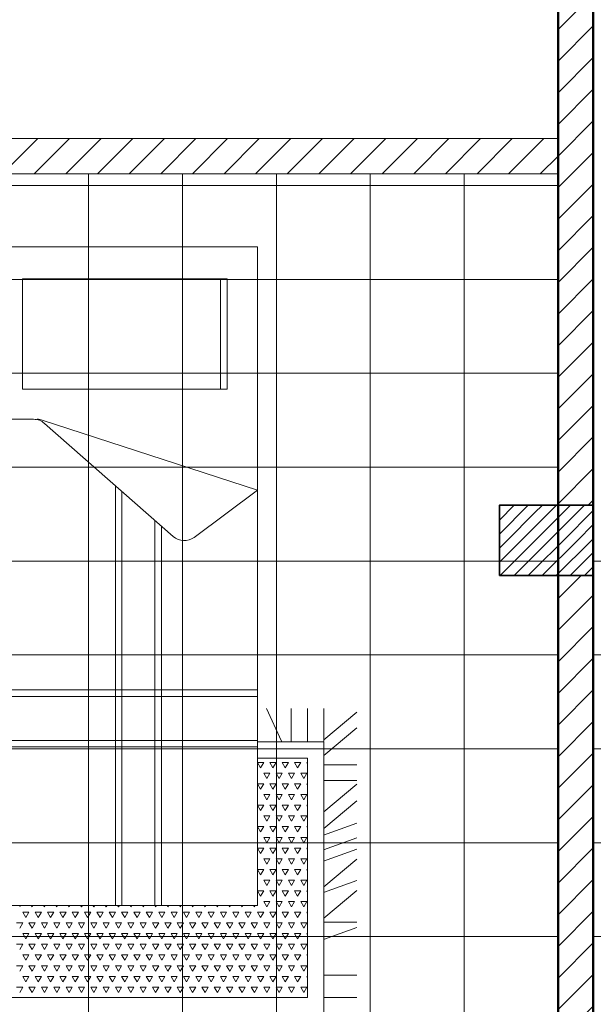
# Model space of a CAD drawing. Units: millimetres. Extents: x 225995 to 227247, y 225507 to 226008.
# Tile 15 of 23: x 226821 to 226894, y 225755 to 225881. Entities that reach past the tile are written whole.
import ezdxf

# ---------------------------------------------------------------- set-up
doc = ezdxf.new("R2010")
doc.units = ezdxf.units.MM
for name, color, linetype, lineweight in [('A-COLS', 40, 'Continuous', 35), ('A-FLOR-PATT', 8, 'Continuous', 13), ('A-FURN', 9, 'Continuous', 18), ('A-WALL', 7, 'Continuous', 50), ('A-WALL-PATT', 8, 'Continuous', 13)]:
    doc.layers.add(name, color=color, linetype=linetype, lineweight=lineweight)
pattern_1 = [(45, (502.0463, 119.0671), (-0.898025612, 0.898025612), [])]

# ---------------------------------------------------------------- blocks, each defined once
blk = doc.blocks.new('A$C6D2A2628')
for p, q in [((0.291, 2.4297), (1.791, 2.4297)), ((1.791, 2.4297), (1.791, 0.4297)), ((1.0779, 2.3321), (1.6991, 2.3321)), ((1.0779, 1.9967), (1.0779, 2.3321)), ((1.6791, 2.3321), (1.6791, 1.9967)), ((1.6991, 2.3321), (1.6991, 1.9967)), ((1.6991, 1.9967), (1.0779, 1.9967)), ((0.9515, 1.9058), (1.1116, 1.9058)), ((1.791, 1.6908), (1.138, 1.9034)), ((1.1446, 1.8934), (1.5358, 1.5497)), ((1.3599, 1.7043), (1.3599, 0.4297)), ((1.3799, 1.6867), (1.3799, 0.4297)), ((1.5987, 1.5472), (1.791, 1.6908)), ((1.4799, 1.5988), (1.4799, 0.4297)), ((1.4999, 1.5812), (1.4999, 0.4297)), ((0.291, 1.0837), (1.791, 1.0837)), ((0.291, 1.0637), (1.791, 1.0637)), ((1.8187, 1.0278), (1.8641, 0.9278)), ((1.8932, 1.0278), (1.8932, 0.9278)), ((1.9432, 1.0278), (1.9432, 0.9278)), ((1.9932, 1.0278), (1.9932, 0.9278)), ((1.9932, 0.9324), (2.0932, 1.016)), ((1.9932, 0.8849), (2.0932, 0.9685)), ((0.291, 0.9307), (1.791, 0.9307)), ((0.291, 0.9107), (1.791, 0.9107)), ((1.9932, 0.9267), (1.791, 0.9267)), ((1.9932, 0.1), (1.9932, 0.9267)), ((1.9432, 0.8767), (1.791, 0.8767)), ((1.9432, 0.15), (1.9432, 0.8767)), ((1.8007, 0.8473), (1.7913, 0.8636)), ((1.7913, 0.8636), (1.8101, 0.8636)), ((1.8007, 0.8473), (1.8101, 0.8636)), ((1.8382, 0.8473), (1.8288, 0.8636)), ((1.8288, 0.8636), (1.8476, 0.8636)), ((1.8382, 0.8473), (1.8476, 0.8636)), ((1.8757, 0.8473), (1.8663, 0.8636)), ((1.8663, 0.8636), (1.8851, 0.8636)), ((1.8757, 0.8473), (1.8851, 0.8636)), ((1.9132, 0.8473), (1.9038, 0.8636)), ((1.9038, 0.8636), (1.9226, 0.8636)), ((1.9132, 0.8473), (1.9226, 0.8636)), ((1.9432, 0.8604), (1.9413, 0.8636)), ((1.9413, 0.8636), (1.9432, 0.8636)), ((1.9932, 0.8564), (2.0932, 0.8564)), ((1.791, 0.8305), (1.7913, 0.8311)), ((1.791, 0.8311), (1.7913, 0.8311)), ((1.8195, 0.8148), (1.8101, 0.8311)), ((1.8101, 0.8311), (1.8288, 0.8311)), ((1.8195, 0.8148), (1.8288, 0.8311)), ((1.857, 0.8148), (1.8476, 0.8311)), ((1.8476, 0.8311), (1.8663, 0.8311)), ((1.857, 0.8148), (1.8663, 0.8311)), ((1.8945, 0.8148), (1.8851, 0.8311)), ((1.8851, 0.8311), (1.9038, 0.8311)), ((1.8945, 0.8148), (1.9038, 0.8311)), ((1.932, 0.8148), (1.9226, 0.8311)), ((1.9226, 0.8311), (1.9413, 0.8311)), ((1.932, 0.8148), (1.9413, 0.8311)), ((1.9932, 0.8089), (2.0932, 0.8089)), ((1.8007, 0.7824), (1.7913, 0.7986)), ((1.7913, 0.7986), (1.8101, 0.7986)), ((1.8007, 0.7824), (1.8101, 0.7986)), ((1.8382, 0.7824), (1.8288, 0.7986)), ((1.8288, 0.7986), (1.8476, 0.7986)), ((1.8382, 0.7824), (1.8476, 0.7986)), ((1.8757, 0.7824), (1.8663, 0.7986)), ((1.8663, 0.7986), (1.8851, 0.7986)), ((1.8757, 0.7824), (1.8851, 0.7986)), ((1.9132, 0.7824), (1.9038, 0.7986)), ((1.9038, 0.7986), (1.9226, 0.7986)), ((1.9132, 0.7824), (1.9226, 0.7986)), ((1.9432, 0.7955), (1.9413, 0.7986)), ((1.9413, 0.7986), (1.9432, 0.7986)), ((1.9932, 0.7139), (2.0932, 0.7975)), ((1.791, 0.7655), (1.7913, 0.7661)), ((1.791, 0.7661), (1.7913, 0.7661)), ((1.8195, 0.7499), (1.8101, 0.7661)), ((1.8101, 0.7661), (1.8288, 0.7661)), ((1.8195, 0.7499), (1.8288, 0.7661)), ((1.857, 0.7499), (1.8476, 0.7661)), ((1.8476, 0.7661), (1.8663, 0.7661)), ((1.857, 0.7499), (1.8663, 0.7661)), ((1.8945, 0.7499), (1.8851, 0.7661)), ((1.8851, 0.7661), (1.9038, 0.7661)), ((1.8945, 0.7499), (1.9038, 0.7661)), ((1.932, 0.7499), (1.9226, 0.7661)), ((1.9226, 0.7661), (1.9413, 0.7661)), ((1.932, 0.7499), (1.9413, 0.7661)), ((1.8007, 0.7174), (1.7913, 0.7337)), ((1.7913, 0.7337), (1.8101, 0.7337)), ((1.8007, 0.7174), (1.8101, 0.7337)), ((1.8382, 0.7174), (1.8288, 0.7337)), ((1.8288, 0.7337), (1.8476, 0.7337)), ((1.8382, 0.7174), (1.8476, 0.7337)), ((1.8757, 0.7174), (1.8663, 0.7337)), ((1.8663, 0.7337), (1.8851, 0.7337)), ((1.8757, 0.7174), (1.8851, 0.7337)), ((1.9132, 0.7174), (1.9038, 0.7337)), ((1.9038, 0.7337), (1.9226, 0.7337)), ((1.9132, 0.7174), (1.9226, 0.7337)), ((1.9432, 0.7305), (1.9413, 0.7337)), ((1.9413, 0.7337), (1.9432, 0.7337)), ((1.9932, 0.6633), (2.0932, 0.7469)), ((1.791, 0.7006), (1.7913, 0.7012)), ((1.791, 0.7012), (1.7913, 0.7012)), ((1.8195, 0.6849), (1.8101, 0.7012)), ((1.8101, 0.7012), (1.8288, 0.7012)), ((1.8195, 0.6849), (1.8288, 0.7012)), ((1.857, 0.6849), (1.8476, 0.7012)), ((1.8476, 0.7012), (1.8663, 0.7012)), ((1.857, 0.6849), (1.8663, 0.7012)), ((1.8945, 0.6849), (1.8851, 0.7012)), ((1.8851, 0.7012), (1.9038, 0.7012)), ((1.8945, 0.6849), (1.9038, 0.7012)), ((1.932, 0.6849), (1.9226, 0.7012)), ((1.9226, 0.7012), (1.9413, 0.7012)), ((1.932, 0.6849), (1.9413, 0.7012)), ((1.8007, 0.6525), (1.7913, 0.6687)), ((1.7913, 0.6687), (1.8101, 0.6687)), ((1.8007, 0.6525), (1.8101, 0.6687)), ((1.8382, 0.6525), (1.8288, 0.6687)), ((1.8288, 0.6687), (1.8476, 0.6687)), ((1.8382, 0.6525), (1.8476, 0.6687)), ((1.8757, 0.6525), (1.8663, 0.6687)), ((1.8663, 0.6687), (1.8851, 0.6687)), ((1.8757, 0.6525), (1.8851, 0.6687)), ((1.9132, 0.6525), (1.9038, 0.6687)), ((1.9038, 0.6687), (1.9226, 0.6687)), ((1.9132, 0.6525), (1.9226, 0.6687)), ((1.9432, 0.6655), (1.9413, 0.6687)), ((1.9413, 0.6687), (1.9432, 0.6687)), ((1.9917, 0.6428), (2.0932, 0.6794)), ((1.791, 0.6356), (1.7913, 0.6362)), ((1.791, 0.6362), (1.7913, 0.6362)), ((1.8195, 0.62), (1.8101, 0.6362)), ((1.8101, 0.6362), (1.8288, 0.6362)), ((1.8195, 0.62), (1.8288, 0.6362)), ((1.857, 0.62), (1.8476, 0.6362)), ((1.8476, 0.6362), (1.8663, 0.6362)), ((1.857, 0.62), (1.8663, 0.6362)), ((1.8945, 0.62), (1.8851, 0.6362)), ((1.8851, 0.6362), (1.9038, 0.6362)), ((1.8945, 0.62), (1.9038, 0.6362)), ((1.932, 0.62), (1.9226, 0.6362)), ((1.9226, 0.6362), (1.9413, 0.6362)), ((1.932, 0.62), (1.9413, 0.6362)), ((1.9917, 0.5984), (2.0932, 0.6351)), ((1.8007, 0.5875), (1.7913, 0.6037)), ((1.7913, 0.6037), (1.8101, 0.6037)), ((1.8007, 0.5875), (1.8101, 0.6037)), ((1.8382, 0.5875), (1.8288, 0.6037)), ((1.8288, 0.6037), (1.8476, 0.6037)), ((1.8382, 0.5875), (1.8476, 0.6037)), ((1.8757, 0.5875), (1.8663, 0.6037)), ((1.8663, 0.6037), (1.8851, 0.6037)), ((1.8757, 0.5875), (1.8851, 0.6037)), ((1.9132, 0.5875), (1.9038, 0.6037)), ((1.9038, 0.6037), (1.9226, 0.6037)), ((1.9132, 0.5875), (1.9226, 0.6037)), ((1.9432, 0.6006), (1.9413, 0.6037)), ((1.9413, 0.6037), (1.9432, 0.6037)), ((1.9917, 0.5636), (2.0932, 0.6003)), ((1.791, 0.5707), (1.7913, 0.5713)), ((1.791, 0.5713), (1.7913, 0.5713)), ((1.8195, 0.555), (1.8101, 0.5713)), ((1.8101, 0.5713), (1.8288, 0.5713)), ((1.8195, 0.555), (1.8288, 0.5713)), ((1.857, 0.555), (1.8476, 0.5713)), ((1.8476, 0.5713), (1.8663, 0.5713)), ((1.857, 0.555), (1.8663, 0.5713)), ((1.8945, 0.555), (1.8851, 0.5713)), ((1.8851, 0.5713), (1.9038, 0.5713)), ((1.8945, 0.555), (1.9038, 0.5713)), ((1.932, 0.555), (1.9226, 0.5713)), ((1.9226, 0.5713), (1.9413, 0.5713)), ((1.932, 0.555), (1.9413, 0.5713)), ((1.9932, 0.4859), (2.0932, 0.5695)), ((1.8007, 0.5226), (1.7913, 0.5388)), ((1.7913, 0.5388), (1.8101, 0.5388)), ((1.8007, 0.5226), (1.8101, 0.5388)), ((1.8382, 0.5226), (1.8288, 0.5388)), ((1.8288, 0.5388), (1.8476, 0.5388)), ((1.8382, 0.5226), (1.8476, 0.5388)), ((1.8757, 0.5226), (1.8663, 0.5388)), ((1.8663, 0.5388), (1.8851, 0.5388)), ((1.8757, 0.5226), (1.8851, 0.5388)), ((1.9132, 0.5226), (1.9038, 0.5388)), ((1.9038, 0.5388), (1.9226, 0.5388)), ((1.9132, 0.5226), (1.9226, 0.5388)), ((1.9432, 0.5356), (1.9413, 0.5388)), ((1.9413, 0.5388), (1.9432, 0.5388)), ((1.791, 0.5057), (1.7913, 0.5063)), ((1.791, 0.5063), (1.7913, 0.5063)), ((1.8195, 0.4901), (1.8101, 0.5063)), ((1.8101, 0.5063), (1.8288, 0.5063)), ((1.8195, 0.4901), (1.8288, 0.5063)), ((1.857, 0.4901), (1.8476, 0.5063)), ((1.8476, 0.5063), (1.8663, 0.5063)), ((1.857, 0.4901), (1.8663, 0.5063)), ((1.8945, 0.4901), (1.8851, 0.5063)), ((1.8851, 0.5063), (1.9038, 0.5063)), ((1.8945, 0.4901), (1.9038, 0.5063)), ((1.932, 0.4901), (1.9226, 0.5063)), ((1.9226, 0.5063), (1.9413, 0.5063)), ((1.932, 0.4901), (1.9413, 0.5063)), ((1.9917, 0.4686), (2.0932, 0.5053)), ((1.8007, 0.4576), (1.7913, 0.4738)), ((1.7913, 0.4738), (1.8101, 0.4738)), ((1.8007, 0.4576), (1.8101, 0.4738)), ((1.8382, 0.4576), (1.8288, 0.4738)), ((1.8288, 0.4738), (1.8476, 0.4738)), ((1.8382, 0.4576), (1.8476, 0.4738)), ((1.8757, 0.4576), (1.8663, 0.4738)), ((1.8663, 0.4738), (1.8851, 0.4738)), ((1.8757, 0.4576), (1.8851, 0.4738)), ((1.9132, 0.4576), (1.9038, 0.4738)), ((1.9038, 0.4738), (1.9226, 0.4738)), ((1.9132, 0.4576), (1.9226, 0.4738)), ((1.9432, 0.4707), (1.9413, 0.4738)), ((1.9413, 0.4738), (1.9432, 0.4738)), ((1.9932, 0.3909), (2.0932, 0.4745)), ((1.791, 0.4297), (0.291, 0.4297)), ((1.0695, 0.4251), (1.0721, 0.4297)), ((1.107, 0.4251), (1.1043, 0.4297)), ((1.107, 0.4251), (1.1096, 0.4297)), ((1.1445, 0.4251), (1.1418, 0.4297)), ((1.1445, 0.4251), (1.1471, 0.4297)), ((1.182, 0.4251), (1.1793, 0.4297)), ((1.182, 0.4251), (1.1846, 0.4297)), ((1.2195, 0.4251), (1.2168, 0.4297)), ((1.2195, 0.4251), (1.2221, 0.4297)), ((1.257, 0.4251), (1.2543, 0.4297)), ((1.257, 0.4251), (1.2596, 0.4297)), ((1.2945, 0.4251), (1.2918, 0.4297)), ((1.2945, 0.4251), (1.2971, 0.4297)), ((1.332, 0.4251), (1.3293, 0.4297)), ((1.332, 0.4251), (1.3346, 0.4297)), ((1.3695, 0.4251), (1.3668, 0.4297)), ((1.3695, 0.4251), (1.3721, 0.4297)), ((1.407, 0.4251), (1.4043, 0.4297)), ((1.407, 0.4251), (1.4096, 0.4297)), ((1.4445, 0.4251), (1.4418, 0.4297)), ((1.4445, 0.4251), (1.4471, 0.4297)), ((1.482, 0.4251), (1.4793, 0.4297)), ((1.482, 0.4251), (1.4846, 0.4297)), ((1.5195, 0.4251), (1.5168, 0.4297)), ((1.5195, 0.4251), (1.5221, 0.4297)), ((1.557, 0.4251), (1.5543, 0.4297)), ((1.557, 0.4251), (1.5596, 0.4297)), ((1.5945, 0.4251), (1.5918, 0.4297)), ((1.5945, 0.4251), (1.5971, 0.4297)), ((1.632, 0.4251), (1.6293, 0.4297)), ((1.632, 0.4251), (1.6346, 0.4297)), ((1.6695, 0.4251), (1.6668, 0.4297)), ((1.6695, 0.4251), (1.6721, 0.4297)), ((1.707, 0.4251), (1.7043, 0.4297)), ((1.707, 0.4251), (1.7096, 0.4297)), ((1.7445, 0.4251), (1.7418, 0.4297)), ((1.7445, 0.4251), (1.7471, 0.4297)), ((1.782, 0.4251), (1.7793, 0.4297)), ((1.782, 0.4251), (1.7846, 0.4297)), ((1.791, 0.4408), (1.7913, 0.4414)), ((1.791, 0.4414), (1.7913, 0.4414)), ((1.8195, 0.4251), (1.8101, 0.4414)), ((1.8101, 0.4414), (1.8288, 0.4414)), ((1.8195, 0.4251), (1.8288, 0.4414)), ((1.857, 0.4251), (1.8476, 0.4414)), ((1.8476, 0.4414), (1.8663, 0.4414)), ((1.857, 0.4251), (1.8663, 0.4414)), ((1.8945, 0.4251), (1.8851, 0.4414)), ((1.8851, 0.4414), (1.9038, 0.4414)), ((1.8945, 0.4251), (1.9038, 0.4414)), ((1.932, 0.4251), (1.9226, 0.4414)), ((1.9226, 0.4414), (1.9413, 0.4414)), ((1.932, 0.4251), (1.9413, 0.4414)), ((1.0882, 0.3927), (1.0788, 0.4089)), ((1.0788, 0.4089), (1.0976, 0.4089)), ((1.0882, 0.3927), (1.0976, 0.4089)), ((1.1257, 0.3927), (1.1163, 0.4089)), ((1.1163, 0.4089), (1.1351, 0.4089)), ((1.1257, 0.3927), (1.1351, 0.4089)), ((1.1632, 0.3927), (1.1538, 0.4089)), ((1.1538, 0.4089), (1.1726, 0.4089)), ((1.1632, 0.3927), (1.1726, 0.4089)), ((1.2007, 0.3927), (1.1913, 0.4089)), ((1.1913, 0.4089), (1.2101, 0.4089)), ((1.2007, 0.3927), (1.2101, 0.4089)), ((1.2382, 0.3927), (1.2288, 0.4089)), ((1.2288, 0.4089), (1.2476, 0.4089)), ((1.2382, 0.3927), (1.2476, 0.4089)), ((1.2757, 0.3927), (1.2663, 0.4089)), ((1.2663, 0.4089), (1.2851, 0.4089)), ((1.2757, 0.3927), (1.2851, 0.4089)), ((1.3132, 0.3927), (1.3038, 0.4089)), ((1.3038, 0.4089), (1.3226, 0.4089)), ((1.3132, 0.3927), (1.3226, 0.4089)), ((1.3507, 0.3927), (1.3413, 0.4089)), ((1.3413, 0.4089), (1.3601, 0.4089)), ((1.3507, 0.3927), (1.3601, 0.4089)), ((1.3882, 0.3927), (1.3788, 0.4089)), ((1.3788, 0.4089), (1.3976, 0.4089)), ((1.3882, 0.3927), (1.3976, 0.4089)), ((1.4257, 0.3927), (1.4163, 0.4089)), ((1.4163, 0.4089), (1.4351, 0.4089)), ((1.4257, 0.3927), (1.4351, 0.4089)), ((1.4632, 0.3927), (1.4538, 0.4089)), ((1.4538, 0.4089), (1.4726, 0.4089)), ((1.4632, 0.3927), (1.4726, 0.4089)), ((1.5007, 0.3927), (1.4913, 0.4089)), ((1.4913, 0.4089), (1.5101, 0.4089)), ((1.5007, 0.3927), (1.5101, 0.4089)), ((1.5382, 0.3927), (1.5288, 0.4089)), ((1.5288, 0.4089), (1.5476, 0.4089)), ((1.5382, 0.3927), (1.5476, 0.4089)), ((1.5757, 0.3927), (1.5663, 0.4089)), ((1.5663, 0.4089), (1.5851, 0.4089)), ((1.5757, 0.3927), (1.5851, 0.4089)), ((1.6132, 0.3927), (1.6038, 0.4089)), ((1.6038, 0.4089), (1.6226, 0.4089)), ((1.6132, 0.3927), (1.6226, 0.4089)), ((1.6507, 0.3927), (1.6413, 0.4089)), ((1.6413, 0.4089), (1.6601, 0.4089)), ((1.6507, 0.3927), (1.6601, 0.4089)), ((1.6882, 0.3927), (1.6788, 0.4089)), ((1.6788, 0.4089), (1.6976, 0.4089)), ((1.6882, 0.3927), (1.6976, 0.4089)), ((1.7257, 0.3927), (1.7163, 0.4089)), ((1.7163, 0.4089), (1.7351, 0.4089)), ((1.7257, 0.3927), (1.7351, 0.4089)), ((1.7632, 0.3927), (1.7538, 0.4089)), ((1.7538, 0.4089), (1.7726, 0.4089)), ((1.7632, 0.3927), (1.7726, 0.4089)), ((1.8007, 0.3927), (1.7913, 0.4089)), ((1.7913, 0.4089), (1.8101, 0.4089)), ((1.8007, 0.3927), (1.8101, 0.4089)), ((1.8382, 0.3927), (1.8288, 0.4089)), ((1.8288, 0.4089), (1.8476, 0.4089)), ((1.8382, 0.3927), (1.8476, 0.4089)), ((1.8757, 0.3927), (1.8663, 0.4089)), ((1.8663, 0.4089), (1.8851, 0.4089)), ((1.8757, 0.3927), (1.8851, 0.4089)), ((1.9132, 0.3927), (1.9038, 0.4089)), ((1.9038, 0.4089), (1.9226, 0.4089)), ((1.9132, 0.3927), (1.9226, 0.4089)), ((1.9432, 0.4057), (1.9413, 0.4089)), ((1.9413, 0.4089), (1.9432, 0.4089)), ((1.0601, 0.3764), (1.0788, 0.3764)), ((1.0695, 0.3602), (1.0788, 0.3764)), ((1.107, 0.3602), (1.0976, 0.3764)), ((1.0976, 0.3764), (1.1163, 0.3764)), ((1.107, 0.3602), (1.1163, 0.3764)), ((1.1445, 0.3602), (1.1351, 0.3764)), ((1.1351, 0.3764), (1.1538, 0.3764)), ((1.1445, 0.3602), (1.1538, 0.3764)), ((1.182, 0.3602), (1.1726, 0.3764)), ((1.1726, 0.3764), (1.1913, 0.3764)), ((1.182, 0.3602), (1.1913, 0.3764)), ((1.2195, 0.3602), (1.2101, 0.3764)), ((1.2101, 0.3764), (1.2288, 0.3764)), ((1.2195, 0.3602), (1.2288, 0.3764)), ((1.257, 0.3602), (1.2476, 0.3764)), ((1.2476, 0.3764), (1.2663, 0.3764)), ((1.257, 0.3602), (1.2663, 0.3764)), ((1.2945, 0.3602), (1.2851, 0.3764)), ((1.2851, 0.3764), (1.3038, 0.3764)), ((1.2945, 0.3602), (1.3038, 0.3764)), ((1.332, 0.3602), (1.3226, 0.3764)), ((1.3226, 0.3764), (1.3413, 0.3764)), ((1.332, 0.3602), (1.3413, 0.3764)), ((1.3695, 0.3602), (1.3601, 0.3764)), ((1.3601, 0.3764), (1.3788, 0.3764)), ((1.3695, 0.3602), (1.3788, 0.3764)), ((1.407, 0.3602), (1.3976, 0.3764)), ((1.3976, 0.3764), (1.4163, 0.3764)), ((1.407, 0.3602), (1.4163, 0.3764)), ((1.4445, 0.3602), (1.4351, 0.3764)), ((1.4351, 0.3764), (1.4538, 0.3764)), ((1.4445, 0.3602), (1.4538, 0.3764)), ((1.482, 0.3602), (1.4726, 0.3764)), ((1.4726, 0.3764), (1.4913, 0.3764)), ((1.482, 0.3602), (1.4913, 0.3764)), ((1.5195, 0.3602), (1.5101, 0.3764)), ((1.5101, 0.3764), (1.5288, 0.3764)), ((1.5195, 0.3602), (1.5288, 0.3764)), ((1.557, 0.3602), (1.5476, 0.3764)), ((1.5476, 0.3764), (1.5663, 0.3764)), ((1.557, 0.3602), (1.5663, 0.3764)), ((1.5945, 0.3602), (1.5851, 0.3764)), ((1.5851, 0.3764), (1.6038, 0.3764)), ((1.5945, 0.3602), (1.6038, 0.3764)), ((1.632, 0.3602), (1.6226, 0.3764)), ((1.6226, 0.3764), (1.6413, 0.3764)), ((1.632, 0.3602), (1.6413, 0.3764)), ((1.6695, 0.3602), (1.6601, 0.3764)), ((1.6601, 0.3764), (1.6788, 0.3764)), ((1.6695, 0.3602), (1.6788, 0.3764)), ((1.707, 0.3602), (1.6976, 0.3764)), ((1.6976, 0.3764), (1.7163, 0.3764)), ((1.707, 0.3602), (1.7163, 0.3764)), ((1.7445, 0.3602), (1.7351, 0.3764)), ((1.7351, 0.3764), (1.7538, 0.3764)), ((1.7445, 0.3602), (1.7538, 0.3764)), ((1.782, 0.3602), (1.7726, 0.3764)), ((1.7726, 0.3764), (1.7913, 0.3764)), ((1.782, 0.3602), (1.7913, 0.3764)), ((1.8195, 0.3602), (1.8101, 0.3764)), ((1.8101, 0.3764), (1.8288, 0.3764)), ((1.8195, 0.3602), (1.8288, 0.3764)), ((1.857, 0.3602), (1.8476, 0.3764)), ((1.8476, 0.3764), (1.8663, 0.3764)), ((1.857, 0.3602), (1.8663, 0.3764)), ((1.8945, 0.3602), (1.8851, 0.3764)), ((1.8851, 0.3764), (1.9038, 0.3764)), ((1.8945, 0.3602), (1.9038, 0.3764)), ((1.932, 0.3602), (1.9226, 0.3764)), ((1.9226, 0.3764), (1.9413, 0.3764)), ((1.932, 0.3602), (1.9413, 0.3764)), ((1.9917, 0.3261), (2.0932, 0.3628)), ((1.9932, 0.3783), (2.0932, 0.3783)), ((1.0882, 0.3277), (1.0788, 0.3439)), ((1.0788, 0.3439), (1.0976, 0.3439)), ((1.0882, 0.3277), (1.0976, 0.3439)), ((1.1257, 0.3277), (1.1163, 0.3439)), ((1.1163, 0.3439), (1.1351, 0.3439)), ((1.1257, 0.3277), (1.1351, 0.3439)), ((1.1632, 0.3277), (1.1538, 0.3439)), ((1.1538, 0.3439), (1.1726, 0.3439)), ((1.1632, 0.3277), (1.1726, 0.3439)), ((1.2007, 0.3277), (1.1913, 0.3439)), ((1.1913, 0.3439), (1.2101, 0.3439)), ((1.2007, 0.3277), (1.2101, 0.3439)), ((1.2382, 0.3277), (1.2288, 0.3439)), ((1.2288, 0.3439), (1.2476, 0.3439)), ((1.2382, 0.3277), (1.2476, 0.3439)), ((1.2757, 0.3277), (1.2663, 0.3439)), ((1.2663, 0.3439), (1.2851, 0.3439)), ((1.2757, 0.3277), (1.2851, 0.3439)), ((1.3132, 0.3277), (1.3038, 0.3439)), ((1.3038, 0.3439), (1.3226, 0.3439)), ((1.3132, 0.3277), (1.3226, 0.3439)), ((1.3507, 0.3277), (1.3413, 0.3439)), ((1.3413, 0.3439), (1.3601, 0.3439)), ((1.3507, 0.3277), (1.3601, 0.3439)), ((1.3882, 0.3277), (1.3788, 0.3439)), ((1.3788, 0.3439), (1.3976, 0.3439)), ((1.3882, 0.3277), (1.3976, 0.3439)), ((1.4257, 0.3277), (1.4163, 0.3439)), ((1.4163, 0.3439), (1.4351, 0.3439)), ((1.4257, 0.3277), (1.4351, 0.3439)), ((1.4632, 0.3277), (1.4538, 0.3439)), ((1.4538, 0.3439), (1.4726, 0.3439)), ((1.4632, 0.3277), (1.4726, 0.3439)), ((1.5007, 0.3277), (1.4913, 0.3439)), ((1.4913, 0.3439), (1.5101, 0.3439)), ((1.5007, 0.3277), (1.5101, 0.3439)), ((1.5382, 0.3277), (1.5288, 0.3439)), ((1.5288, 0.3439), (1.5476, 0.3439)), ((1.5382, 0.3277), (1.5476, 0.3439)), ((1.5757, 0.3277), (1.5663, 0.3439)), ((1.5663, 0.3439), (1.5851, 0.3439)), ((1.5757, 0.3277), (1.5851, 0.3439)), ((1.6132, 0.3277), (1.6038, 0.3439)), ((1.6038, 0.3439), (1.6226, 0.3439)), ((1.6132, 0.3277), (1.6226, 0.3439)), ((1.6507, 0.3277), (1.6413, 0.3439)), ((1.6413, 0.3439), (1.6601, 0.3439)), ((1.6507, 0.3277), (1.6601, 0.3439)), ((1.6882, 0.3277), (1.6788, 0.3439)), ((1.6788, 0.3439), (1.6976, 0.3439)), ((1.6882, 0.3277), (1.6976, 0.3439)), ((1.7257, 0.3277), (1.7163, 0.3439)), ((1.7163, 0.3439), (1.7351, 0.3439)), ((1.7257, 0.3277), (1.7351, 0.3439)), ((1.7632, 0.3277), (1.7538, 0.3439)), ((1.7538, 0.3439), (1.7726, 0.3439)), ((1.7632, 0.3277), (1.7726, 0.3439)), ((1.8007, 0.3277), (1.7913, 0.3439)), ((1.7913, 0.3439), (1.8101, 0.3439)), ((1.8007, 0.3277), (1.8101, 0.3439)), ((1.8382, 0.3277), (1.8288, 0.3439)), ((1.8288, 0.3439), (1.8476, 0.3439)), ((1.8382, 0.3277), (1.8476, 0.3439)), ((1.8757, 0.3277), (1.8663, 0.3439)), ((1.8663, 0.3439), (1.8851, 0.3439)), ((1.8757, 0.3277), (1.8851, 0.3439)), ((1.9132, 0.3277), (1.9038, 0.3439)), ((1.9038, 0.3439), (1.9226, 0.3439)), ((1.9132, 0.3277), (1.9226, 0.3439)), ((1.9432, 0.3408), (1.9413, 0.3439)), ((1.9413, 0.3439), (1.9432, 0.3439)), ((1.0601, 0.3115), (1.0788, 0.3115)), ((1.0695, 0.2952), (1.0788, 0.3115)), ((1.107, 0.2952), (1.0976, 0.3115)), ((1.0976, 0.3115), (1.1163, 0.3115)), ((1.107, 0.2952), (1.1163, 0.3115)), ((1.1445, 0.2952), (1.1351, 0.3115)), ((1.1351, 0.3115), (1.1538, 0.3115)), ((1.1445, 0.2952), (1.1538, 0.3115)), ((1.182, 0.2952), (1.1726, 0.3115)), ((1.1726, 0.3115), (1.1913, 0.3115)), ((1.182, 0.2952), (1.1913, 0.3115)), ((1.2195, 0.2952), (1.2101, 0.3115)), ((1.2101, 0.3115), (1.2288, 0.3115)), ((1.2195, 0.2952), (1.2288, 0.3115)), ((1.257, 0.2952), (1.2476, 0.3115)), ((1.2476, 0.3115), (1.2663, 0.3115)), ((1.257, 0.2952), (1.2663, 0.3115)), ((1.2945, 0.2952), (1.2851, 0.3115)), ((1.2851, 0.3115), (1.3038, 0.3115)), ((1.2945, 0.2952), (1.3038, 0.3115)), ((1.332, 0.2952), (1.3226, 0.3115)), ((1.3226, 0.3115), (1.3413, 0.3115)), ((1.332, 0.2952), (1.3413, 0.3115)), ((1.3695, 0.2952), (1.3601, 0.3115)), ((1.3601, 0.3115), (1.3788, 0.3115)), ((1.3695, 0.2952), (1.3788, 0.3115)), ((1.407, 0.2952), (1.3976, 0.3115)), ((1.3976, 0.3115), (1.4163, 0.3115)), ((1.407, 0.2952), (1.4163, 0.3115)), ((1.4445, 0.2952), (1.4351, 0.3115)), ((1.4351, 0.3115), (1.4538, 0.3115)), ((1.4445, 0.2952), (1.4538, 0.3115)), ((1.482, 0.2952), (1.4726, 0.3115)), ((1.4726, 0.3115), (1.4913, 0.3115)), ((1.482, 0.2952), (1.4913, 0.3115)), ((1.5195, 0.2952), (1.5101, 0.3115)), ((1.5101, 0.3115), (1.5288, 0.3115)), ((1.5195, 0.2952), (1.5288, 0.3115)), ((1.557, 0.2952), (1.5476, 0.3115)), ((1.5476, 0.3115), (1.5663, 0.3115)), ((1.557, 0.2952), (1.5663, 0.3115)), ((1.5945, 0.2952), (1.5851, 0.3115)), ((1.5851, 0.3115), (1.6038, 0.3115)), ((1.5945, 0.2952), (1.6038, 0.3115)), ((1.632, 0.2952), (1.6226, 0.3115)), ((1.6226, 0.3115), (1.6413, 0.3115)), ((1.632, 0.2952), (1.6413, 0.3115)), ((1.6695, 0.2952), (1.6601, 0.3115)), ((1.6601, 0.3115), (1.6788, 0.3115)), ((1.6695, 0.2952), (1.6788, 0.3115)), ((1.707, 0.2952), (1.6976, 0.3115)), ((1.6976, 0.3115), (1.7163, 0.3115)), ((1.707, 0.2952), (1.7163, 0.3115)), ((1.7445, 0.2952), (1.7351, 0.3115)), ((1.7351, 0.3115), (1.7538, 0.3115)), ((1.7445, 0.2952), (1.7538, 0.3115)), ((1.782, 0.2952), (1.7726, 0.3115)), ((1.7726, 0.3115), (1.7913, 0.3115)), ((1.782, 0.2952), (1.7913, 0.3115)), ((1.8195, 0.2952), (1.8101, 0.3115)), ((1.8101, 0.3115), (1.8288, 0.3115)), ((1.8195, 0.2952), (1.8288, 0.3115)), ((1.857, 0.2952), (1.8476, 0.3115)), ((1.8476, 0.3115), (1.8663, 0.3115)), ((1.857, 0.2952), (1.8663, 0.3115)), ((1.8945, 0.2952), (1.8851, 0.3115)), ((1.8851, 0.3115), (1.9038, 0.3115)), ((1.8945, 0.2952), (1.9038, 0.3115)), ((1.932, 0.2952), (1.9226, 0.3115)), ((1.9226, 0.3115), (1.9413, 0.3115)), ((1.932, 0.2952), (1.9413, 0.3115)), ((1.0882, 0.2628), (1.0788, 0.279)), ((1.0788, 0.279), (1.0976, 0.279)), ((1.0882, 0.2628), (1.0976, 0.279)), ((1.1257, 0.2628), (1.1163, 0.279)), ((1.1163, 0.279), (1.1351, 0.279)), ((1.1257, 0.2628), (1.1351, 0.279)), ((1.1632, 0.2628), (1.1538, 0.279)), ((1.1538, 0.279), (1.1726, 0.279)), ((1.1632, 0.2628), (1.1726, 0.279)), ((1.2007, 0.2628), (1.1913, 0.279)), ((1.1913, 0.279), (1.2101, 0.279)), ((1.2007, 0.2628), (1.2101, 0.279)), ((1.2382, 0.2628), (1.2288, 0.279)), ((1.2288, 0.279), (1.2476, 0.279)), ((1.2382, 0.2628), (1.2476, 0.279)), ((1.2757, 0.2628), (1.2663, 0.279)), ((1.2663, 0.279), (1.2851, 0.279)), ((1.2757, 0.2628), (1.2851, 0.279)), ((1.3132, 0.2628), (1.3038, 0.279)), ((1.3038, 0.279), (1.3226, 0.279)), ((1.3132, 0.2628), (1.3226, 0.279)), ((1.3507, 0.2628), (1.3413, 0.279)), ((1.3413, 0.279), (1.3601, 0.279)), ((1.3507, 0.2628), (1.3601, 0.279)), ((1.3882, 0.2628), (1.3788, 0.279)), ((1.3788, 0.279), (1.3976, 0.279)), ((1.3882, 0.2628), (1.3976, 0.279)), ((1.4257, 0.2628), (1.4163, 0.279)), ((1.4163, 0.279), (1.4351, 0.279)), ((1.4257, 0.2628), (1.4351, 0.279)), ((1.4632, 0.2628), (1.4538, 0.279)), ((1.4538, 0.279), (1.4726, 0.279)), ((1.4632, 0.2628), (1.4726, 0.279)), ((1.5007, 0.2628), (1.4913, 0.279)), ((1.4913, 0.279), (1.5101, 0.279)), ((1.5007, 0.2628), (1.5101, 0.279)), ((1.5382, 0.2628), (1.5288, 0.279)), ((1.5288, 0.279), (1.5476, 0.279)), ((1.5382, 0.2628), (1.5476, 0.279)), ((1.5757, 0.2628), (1.5663, 0.279)), ((1.5663, 0.279), (1.5851, 0.279)), ((1.5757, 0.2628), (1.5851, 0.279)), ((1.6132, 0.2628), (1.6038, 0.279)), ((1.6038, 0.279), (1.6226, 0.279)), ((1.6132, 0.2628), (1.6226, 0.279)), ((1.6507, 0.2628), (1.6413, 0.279)), ((1.6413, 0.279), (1.6601, 0.279)), ((1.6507, 0.2628), (1.6601, 0.279)), ((1.6882, 0.2628), (1.6788, 0.279)), ((1.6788, 0.279), (1.6976, 0.279)), ((1.6882, 0.2628), (1.6976, 0.279)), ((1.7257, 0.2628), (1.7163, 0.279)), ((1.7163, 0.279), (1.7351, 0.279)), ((1.7257, 0.2628), (1.7351, 0.279)), ((1.7632, 0.2628), (1.7538, 0.279)), ((1.7538, 0.279), (1.7726, 0.279)), ((1.7632, 0.2628), (1.7726, 0.279)), ((1.8007, 0.2628), (1.7913, 0.279)), ((1.7913, 0.279), (1.8101, 0.279)), ((1.8007, 0.2628), (1.8101, 0.279)), ((1.8382, 0.2628), (1.8288, 0.279)), ((1.8288, 0.279), (1.8476, 0.279)), ((1.8382, 0.2628), (1.8476, 0.279)), ((1.8757, 0.2628), (1.8663, 0.279)), ((1.8663, 0.279), (1.8851, 0.279)), ((1.8757, 0.2628), (1.8851, 0.279)), ((1.9132, 0.2628), (1.9038, 0.279)), ((1.9038, 0.279), (1.9226, 0.279)), ((1.9132, 0.2628), (1.9226, 0.279)), ((1.9432, 0.2758), (1.9413, 0.279)), ((1.9413, 0.279), (1.9432, 0.279)), ((1.0601, 0.2465), (1.0788, 0.2465)), ((1.0695, 0.2303), (1.0788, 0.2465)), ((1.107, 0.2303), (1.0976, 0.2465)), ((1.0976, 0.2465), (1.1163, 0.2465)), ((1.107, 0.2303), (1.1163, 0.2465)), ((1.1445, 0.2303), (1.1351, 0.2465)), ((1.1351, 0.2465), (1.1538, 0.2465)), ((1.1445, 0.2303), (1.1538, 0.2465)), ((1.182, 0.2303), (1.1726, 0.2465)), ((1.1726, 0.2465), (1.1913, 0.2465)), ((1.182, 0.2303), (1.1913, 0.2465)), ((1.2195, 0.2303), (1.2101, 0.2465)), ((1.2101, 0.2465), (1.2288, 0.2465)), ((1.2195, 0.2303), (1.2288, 0.2465)), ((1.257, 0.2303), (1.2476, 0.2465)), ((1.2476, 0.2465), (1.2663, 0.2465)), ((1.257, 0.2303), (1.2663, 0.2465)), ((1.2945, 0.2303), (1.2851, 0.2465)), ((1.2851, 0.2465), (1.3038, 0.2465)), ((1.2945, 0.2303), (1.3038, 0.2465)), ((1.332, 0.2303), (1.3226, 0.2465)), ((1.3226, 0.2465), (1.3413, 0.2465)), ((1.332, 0.2303), (1.3413, 0.2465)), ((1.3695, 0.2303), (1.3601, 0.2465)), ((1.3601, 0.2465), (1.3788, 0.2465)), ((1.3695, 0.2303), (1.3788, 0.2465)), ((1.407, 0.2303), (1.3976, 0.2465)), ((1.3976, 0.2465), (1.4163, 0.2465)), ((1.407, 0.2303), (1.4163, 0.2465)), ((1.4445, 0.2303), (1.4351, 0.2465)), ((1.4351, 0.2465), (1.4538, 0.2465)), ((1.4445, 0.2303), (1.4538, 0.2465)), ((1.482, 0.2303), (1.4726, 0.2465)), ((1.4726, 0.2465), (1.4913, 0.2465)), ((1.482, 0.2303), (1.4913, 0.2465)), ((1.5195, 0.2303), (1.5101, 0.2465)), ((1.5101, 0.2465), (1.5288, 0.2465)), ((1.5195, 0.2303), (1.5288, 0.2465)), ((1.557, 0.2303), (1.5476, 0.2465)), ((1.5476, 0.2465), (1.5663, 0.2465)), ((1.557, 0.2303), (1.5663, 0.2465)), ((1.5945, 0.2303), (1.5851, 0.2465)), ((1.5851, 0.2465), (1.6038, 0.2465)), ((1.5945, 0.2303), (1.6038, 0.2465)), ((1.632, 0.2303), (1.6226, 0.2465)), ((1.6226, 0.2465), (1.6413, 0.2465)), ((1.632, 0.2303), (1.6413, 0.2465)), ((1.6695, 0.2303), (1.6601, 0.2465)), ((1.6601, 0.2465), (1.6788, 0.2465)), ((1.6695, 0.2303), (1.6788, 0.2465)), ((1.707, 0.2303), (1.6976, 0.2465)), ((1.6976, 0.2465), (1.7163, 0.2465)), ((1.707, 0.2303), (1.7163, 0.2465)), ((1.7445, 0.2303), (1.7351, 0.2465)), ((1.7351, 0.2465), (1.7538, 0.2465)), ((1.7445, 0.2303), (1.7538, 0.2465)), ((1.782, 0.2303), (1.7726, 0.2465)), ((1.7726, 0.2465), (1.7913, 0.2465)), ((1.782, 0.2303), (1.7913, 0.2465)), ((1.8195, 0.2303), (1.8101, 0.2465)), ((1.8101, 0.2465), (1.8288, 0.2465)), ((1.8195, 0.2303), (1.8288, 0.2465)), ((1.857, 0.2303), (1.8476, 0.2465)), ((1.8476, 0.2465), (1.8663, 0.2465)), ((1.857, 0.2303), (1.8663, 0.2465)), ((1.8945, 0.2303), (1.8851, 0.2465)), ((1.8851, 0.2465), (1.9038, 0.2465)), ((1.8945, 0.2303), (1.9038, 0.2465)), ((1.932, 0.2303), (1.9226, 0.2465)), ((1.9226, 0.2465), (1.9413, 0.2465)), ((1.932, 0.2303), (1.9413, 0.2465)), ((1.0882, 0.1978), (1.0788, 0.214)), ((1.0788, 0.214), (1.0976, 0.214)), ((1.0882, 0.1978), (1.0976, 0.214)), ((1.1257, 0.1978), (1.1163, 0.214)), ((1.1163, 0.214), (1.1351, 0.214)), ((1.1257, 0.1978), (1.1351, 0.214)), ((1.1632, 0.1978), (1.1538, 0.214)), ((1.1538, 0.214), (1.1726, 0.214)), ((1.1632, 0.1978), (1.1726, 0.214)), ((1.2007, 0.1978), (1.1913, 0.214)), ((1.1913, 0.214), (1.2101, 0.214)), ((1.2007, 0.1978), (1.2101, 0.214)), ((1.2382, 0.1978), (1.2288, 0.214)), ((1.2288, 0.214), (1.2476, 0.214)), ((1.2382, 0.1978), (1.2476, 0.214)), ((1.2757, 0.1978), (1.2663, 0.214)), ((1.2663, 0.214), (1.2851, 0.214)), ((1.2757, 0.1978), (1.2851, 0.214)), ((1.3132, 0.1978), (1.3038, 0.214)), ((1.3038, 0.214), (1.3226, 0.214)), ((1.3132, 0.1978), (1.3226, 0.214)), ((1.3507, 0.1978), (1.3413, 0.214)), ((1.3413, 0.214), (1.3601, 0.214)), ((1.3507, 0.1978), (1.3601, 0.214)), ((1.3882, 0.1978), (1.3788, 0.214)), ((1.3788, 0.214), (1.3976, 0.214)), ((1.3882, 0.1978), (1.3976, 0.214)), ((1.4257, 0.1978), (1.4163, 0.214)), ((1.4163, 0.214), (1.4351, 0.214)), ((1.4257, 0.1978), (1.4351, 0.214)), ((1.4632, 0.1978), (1.4538, 0.214)), ((1.4538, 0.214), (1.4726, 0.214)), ((1.4632, 0.1978), (1.4726, 0.214)), ((1.5007, 0.1978), (1.4913, 0.214)), ((1.4913, 0.214), (1.5101, 0.214)), ((1.5007, 0.1978), (1.5101, 0.214)), ((1.5382, 0.1978), (1.5288, 0.214)), ((1.5288, 0.214), (1.5476, 0.214)), ((1.5382, 0.1978), (1.5476, 0.214)), ((1.5757, 0.1978), (1.5663, 0.214)), ((1.5663, 0.214), (1.5851, 0.214)), ((1.5757, 0.1978), (1.5851, 0.214)), ((1.6132, 0.1978), (1.6038, 0.214)), ((1.6038, 0.214), (1.6226, 0.214)), ((1.6132, 0.1978), (1.6226, 0.214)), ((1.6507, 0.1978), (1.6413, 0.214)), ((1.6413, 0.214), (1.6601, 0.214)), ((1.6507, 0.1978), (1.6601, 0.214)), ((1.6882, 0.1978), (1.6788, 0.214)), ((1.6788, 0.214), (1.6976, 0.214)), ((1.6882, 0.1978), (1.6976, 0.214)), ((1.7257, 0.1978), (1.7163, 0.214)), ((1.7163, 0.214), (1.7351, 0.214)), ((1.7257, 0.1978), (1.7351, 0.214)), ((1.7632, 0.1978), (1.7538, 0.214)), ((1.7538, 0.214), (1.7726, 0.214)), ((1.7632, 0.1978), (1.7726, 0.214)), ((1.8007, 0.1978), (1.7913, 0.214)), ((1.7913, 0.214), (1.8101, 0.214)), ((1.8007, 0.1978), (1.8101, 0.214)), ((1.8382, 0.1978), (1.8288, 0.214)), ((1.8288, 0.214), (1.8476, 0.214)), ((1.8382, 0.1978), (1.8476, 0.214)), ((1.8757, 0.1978), (1.8663, 0.214)), ((1.8663, 0.214), (1.8851, 0.214)), ((1.8757, 0.1978), (1.8851, 0.214)), ((1.9132, 0.1978), (1.9038, 0.214)), ((1.9038, 0.214), (1.9226, 0.214)), ((1.9132, 0.1978), (1.9226, 0.214)), ((1.9432, 0.2109), (1.9413, 0.214)), ((1.9413, 0.214), (1.9432, 0.214)), ((1.9932, 0.2173), (2.0932, 0.2173)), ((1.0601, 0.1816), (1.0788, 0.1816)), ((1.0695, 0.1653), (1.0788, 0.1816)), ((1.107, 0.1653), (1.0976, 0.1816)), ((1.0976, 0.1816), (1.1163, 0.1816)), ((1.107, 0.1653), (1.1163, 0.1816)), ((1.1445, 0.1653), (1.1351, 0.1816)), ((1.1351, 0.1816), (1.1538, 0.1816)), ((1.1445, 0.1653), (1.1538, 0.1816)), ((1.182, 0.1653), (1.1726, 0.1816)), ((1.1726, 0.1816), (1.1913, 0.1816)), ((1.182, 0.1653), (1.1913, 0.1816)), ((1.2195, 0.1653), (1.2101, 0.1816)), ((1.2101, 0.1816), (1.2288, 0.1816)), ((1.2195, 0.1653), (1.2288, 0.1816)), ((1.257, 0.1653), (1.2476, 0.1816)), ((1.2476, 0.1816), (1.2663, 0.1816)), ((1.257, 0.1653), (1.2663, 0.1816)), ((1.2945, 0.1653), (1.2851, 0.1816)), ((1.2851, 0.1816), (1.3038, 0.1816)), ((1.2945, 0.1653), (1.3038, 0.1816)), ((1.332, 0.1653), (1.3226, 0.1816)), ((1.3226, 0.1816), (1.3413, 0.1816)), ((1.332, 0.1653), (1.3413, 0.1816)), ((1.3695, 0.1653), (1.3601, 0.1816)), ((1.3601, 0.1816), (1.3788, 0.1816)), ((1.3695, 0.1653), (1.3788, 0.1816)), ((1.407, 0.1653), (1.3976, 0.1816)), ((1.3976, 0.1816), (1.4163, 0.1816)), ((1.407, 0.1653), (1.4163, 0.1816)), ((1.4445, 0.1653), (1.4351, 0.1816)), ((1.4351, 0.1816), (1.4538, 0.1816)), ((1.4445, 0.1653), (1.4538, 0.1816)), ((1.482, 0.1653), (1.4726, 0.1816)), ((1.4726, 0.1816), (1.4913, 0.1816)), ((1.482, 0.1653), (1.4913, 0.1816)), ((1.5195, 0.1653), (1.5101, 0.1816)), ((1.5101, 0.1816), (1.5288, 0.1816)), ((1.5195, 0.1653), (1.5288, 0.1816)), ((1.557, 0.1653), (1.5476, 0.1816)), ((1.5476, 0.1816), (1.5663, 0.1816)), ((1.557, 0.1653), (1.5663, 0.1816)), ((1.5945, 0.1653), (1.5851, 0.1816)), ((1.5851, 0.1816), (1.6038, 0.1816)), ((1.5945, 0.1653), (1.6038, 0.1816)), ((1.632, 0.1653), (1.6226, 0.1816)), ((1.6226, 0.1816), (1.6413, 0.1816)), ((1.632, 0.1653), (1.6413, 0.1816)), ((1.6695, 0.1653), (1.6601, 0.1816)), ((1.6601, 0.1816), (1.6788, 0.1816)), ((1.6695, 0.1653), (1.6788, 0.1816)), ((1.707, 0.1653), (1.6976, 0.1816)), ((1.6976, 0.1816), (1.7163, 0.1816)), ((1.707, 0.1653), (1.7163, 0.1816)), ((1.7445, 0.1653), (1.7351, 0.1816)), ((1.7351, 0.1816), (1.7538, 0.1816)), ((1.7445, 0.1653), (1.7538, 0.1816)), ((1.782, 0.1653), (1.7726, 0.1816)), ((1.7726, 0.1816), (1.7913, 0.1816)), ((1.782, 0.1653), (1.7913, 0.1816)), ((1.8195, 0.1653), (1.8101, 0.1816)), ((1.8101, 0.1816), (1.8288, 0.1816)), ((1.8195, 0.1653), (1.8288, 0.1816)), ((1.857, 0.1653), (1.8476, 0.1816)), ((1.8476, 0.1816), (1.8663, 0.1816)), ((1.857, 0.1653), (1.8663, 0.1816)), ((1.8945, 0.1653), (1.8851, 0.1816)), ((1.8851, 0.1816), (1.9038, 0.1816)), ((1.8945, 0.1653), (1.9038, 0.1816)), ((1.932, 0.1653), (1.9226, 0.1816)), ((1.9226, 0.1816), (1.9413, 0.1816)), ((1.932, 0.1653), (1.9413, 0.1816)), ((0.1519, 0.15), (1.9432, 0.15)), ((1.9932, 0.15), (2.0932, 0.15))]:
    blk.add_line(p, q)
for centre, start, end in [((1.1116, 1.8558), 48.6958, 90), ((1.1225, 1.8558), 71.966, 90), ((1.5688, 1.5873), 228.6958, 306.7579)]:
    blk.add_arc(centre, 0.05, start, end)

msp = doc.modelspace()

# ---------------------------------------------------------------- hatches: boundary and pattern name
at = {"layer": 'A-WALL-PATT'}
h = msp.add_hatch(dxfattribs=at)
h.set_pattern_fill('ANSI31', color=256, scale=0.9)
h.paths.add_polyline_path([(226894.42, 225925.7), (226889.92, 225925.7), (226889.92, 225818.84), (226894.42, 225818.84)])
h = msp.add_hatch(dxfattribs=at)
h.set_pattern_fill('ANSI31', color=256, scale=0.9)
h.paths.add_polyline_path([(226889.92, 225865.7), (226810.42, 225865.7), (226810.42, 225877.21), (226805.92, 225877.21), (226805.92, 225861.2), (226889.92, 225861.2)])
h = msp.add_hatch(dxfattribs=at)
h.set_pattern_fill('ANSI31', color=256, scale=0.4)
h.set_pattern_definition(pattern_1)
h.paths.add_polyline_path([(226886.92, 225818.84), (226882.42, 225818.84), (226882.42, 225814.34), (226886.92, 225814.34)])
h = msp.add_hatch(dxfattribs=at)
h.set_pattern_fill('ANSI31', color=256, scale=0.4)
h.set_pattern_definition(pattern_1)
h.paths.add_polyline_path([(226894.42, 225818.84), (226886.92, 225818.84), (226886.92, 225814.34), (226894.42, 225814.34)])
h = msp.add_hatch(dxfattribs=at)
h.set_pattern_fill('ANSI31', color=256, scale=0.4)
h.set_pattern_definition(pattern_1)
h.paths.add_polyline_path([(226886.92, 225814.34), (226882.42, 225814.34), (226882.42, 225809.84), (226886.92, 225809.84)])
h = msp.add_hatch(dxfattribs=at)
h.set_pattern_fill('ANSI31', color=256, scale=0.4)
h.set_pattern_definition(pattern_1)
h.paths.add_polyline_path([(226894.42, 225814.34), (226886.92, 225814.34), (226886.92, 225809.84), (226894.42, 225809.84)])
h = msp.add_hatch(dxfattribs=at)
h.set_pattern_fill('ANSI31', color=256, scale=0.9)
h.paths.add_polyline_path([(226894.42, 225809.84), (226889.92, 225809.84), (226889.92, 225741.2), (226894.42, 225741.2)])

# ---------------------------------------------------------------- linework, layer by layer
at = {"layer": 'A-COLS'}
msp.add_lwpolyline([(226882.42, 225809.84), (226882.42, 225818.84), (226894.42, 225818.84), (226894.42, 225809.84)], close=True, dxfattribs=at)
at = {"layer": 'A-FLOR-PATT'}
for p, q in [((226829.92, 225861.2), (226829.92, 225700.7)), ((226841.92, 225861.2), (226841.92, 225700.7)), ((226853.92, 225861.2), (226853.92, 225700.7)), ((226865.92, 225861.2), (226865.92, 225700.7)), ((226877.92, 225861.2), (226877.92, 225700.7)), ((226757.92, 225859.7), (226889.92, 225859.7)), ((226757.92, 225847.7), (226889.92, 225847.7)), ((226757.92, 225835.7), (226889.92, 225835.7)), ((226757.92, 225823.7), (226889.92, 225823.7)), ((226757.92, 225811.7), (226889.92, 225811.7)), ((226894.42, 225811.7), (226984.42, 225811.7)), ((226757.92, 225799.7), (226889.92, 225799.7)), ((226894.42, 225799.7), (227026.42, 225799.7)), ((226757.92, 225787.7), (226889.92, 225787.7)), ((226894.42, 225787.7), (227026.42, 225787.7)), ((226757.92, 225775.7), (226889.92, 225775.7)), ((226894.42, 225775.7), (227026.42, 225775.7)), ((226757.92, 225763.7), (226889.92, 225763.7)), ((226894.42, 225763.7), (227026.42, 225763.7))]:
    msp.add_line(p, q, dxfattribs=at)
at = {"layer": 'A-FURN'}
for p, q in [((226810.42, 225865.7), (226889.92, 225865.7)), ((226889.92, 225865.7), (226810.42, 225865.7)), ((226805.92, 225861.2), (226889.92, 225861.2)), ((226805.92, 225861.2), (226889.92, 225861.2)), ((226889.92, 225809.85), (226894.42, 225809.84)), ((226890.09, 225809.85), (226890.09, 225809.84))]:
    msp.add_line(p, q, dxfattribs=at)
at = {"layer": 'A-WALL'}
for p, q in [((226889.92, 225741.2), (226889.92, 225934.7)), ((226889.92, 225741.2), (226889.92, 225925.7)), ((226894.42, 225741.2), (226894.42, 225925.7)), ((226894.42, 225925.7), (226894.42, 225741.2))]:
    msp.add_line(p, q, dxfattribs=at)

# ---------------------------------------------------------------- block references
at = {"layer": 'A-FURN', "xscale": 42.09102840542158, "yscale": 42.09102840542158, "zscale": 42.09102840542158}
msp.add_blockref('A$C6D2A2628', (226776.11, 225749.61), dxfattribs=at)

doc.saveas('drawing.dxf')
